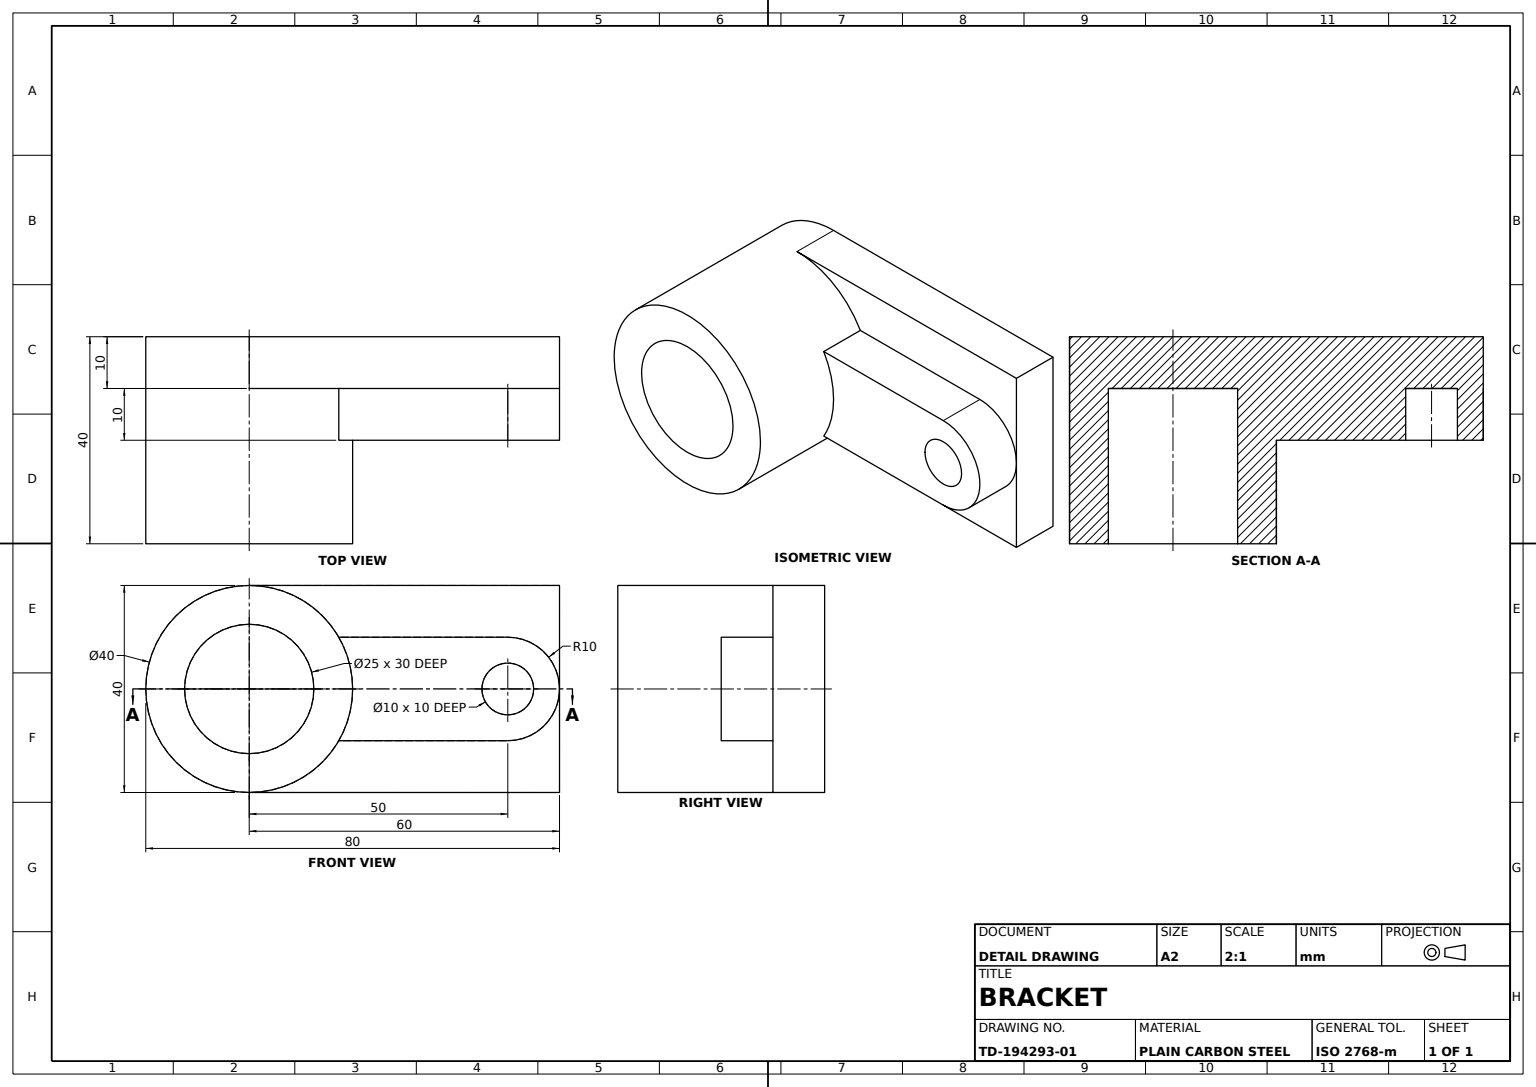
from build123d import *

# Parameters (mm, degrees)
BASE_PLATE_SKETCH_W                = 60
BASE_PLATE_SKETCH_H                = 40
BASE_PLATE_DEPTH                   = 10
CYLINDER_BOSS_SKETCH_40_R          = 20
CYLINDER_BOSS_40_DEPTH             = 40
CYLINDER_ROOT_BOSS_SKETCH_40_R     = 20
CYLINDER_ROOT_BOSS_40_DEPTH        = 10
CYLINDER_START                     = -10
CYLINDER_CLEARANCE_CUT_SKETCH_40_R = 20
CYLINDER_CLEARANCE_CUT_40_DEPTH    = 10
LUG_ARM_DEPTH                      = 10
LUG_HOLE_SKETCH_10_R               = 5
LUG_HOLE_10_DEPTH                  = 10
BORE_SKETCH_25_R                   = 12.5
BORE_25_DEPTH                      = 30


with BuildPart() as part:
    # Base Plate Sketch → Base Plate (new body)
    with BuildSketch(Plane.XY):
        with Locations((30, -20)):
            Rectangle(BASE_PLATE_SKETCH_W, BASE_PLATE_SKETCH_H)
    extrude(amount=BASE_PLATE_DEPTH)

    # Cylinder Boss Sketch Ø40 → Cylinder Boss Ø40 (add)
    with BuildSketch(Plane.XY.offset(10)):
        with Locations(Location((0, -20, 0), (0, 0, 270))):
            Circle(CYLINDER_BOSS_SKETCH_40_R)
    extrude(amount=CYLINDER_BOSS_40_DEPTH)

    # Cylinder Root Boss Sketch Ø40 → Cylinder Root Boss Ø40 (add)
    with BuildSketch(Plane(origin=(0, 0, 0), x_dir=(-1, 0, 0), z_dir=(0, 0, -1))):
        with Locations(Location((0, -20, 0), (0, 0, 90))):
            Circle(CYLINDER_ROOT_BOSS_SKETCH_40_R)
    extrude(amount=-CYLINDER_ROOT_BOSS_40_DEPTH)

    # Cylinder Clearance Cut Sketch Ø40 → Cylinder Clearance Cut Ø40 (cut)
    with BuildSketch(Plane.XY.offset(50).offset(CYLINDER_START)):
        with Locations(Location((0, -20, 0), (0, 0, 90))):
            Circle(CYLINDER_CLEARANCE_CUT_SKETCH_40_R)
    extrude(amount=CYLINDER_CLEARANCE_CUT_40_DEPTH, mode=Mode.SUBTRACT)

    # Lug Arm Sketch → Lug Arm (add)
    with BuildSketch(Plane.XY.offset(10)):
        with BuildLine():
            Line((50, -10), (17.320508076, -10))
            ThreePointArc((17.320508076, -10), (20, -20), (17.320508076, -30))
            Line((17.320508076, -30), (50, -30))
            ThreePointArc((50, -30), (60, -20), (50, -10))
        make_face()
    extrude(amount=LUG_ARM_DEPTH)

    # Lug Hole Sketch Ø10 → Lug Hole Ø10 (cut)
    with BuildSketch(Plane.XY.offset(20)):
        with Locations((50, -20)):
            Circle(LUG_HOLE_SKETCH_10_R)
    extrude(amount=-LUG_HOLE_10_DEPTH, mode=Mode.SUBTRACT)

    # Bore Sketch Ø25 → Bore Ø25 (cut)
    with BuildSketch(Plane.XY.offset(40)):
        with Locations((0, -20)):
            Circle(BORE_SKETCH_25_R)
    extrude(amount=-BORE_25_DEPTH, mode=Mode.SUBTRACT)


solid = part.part
